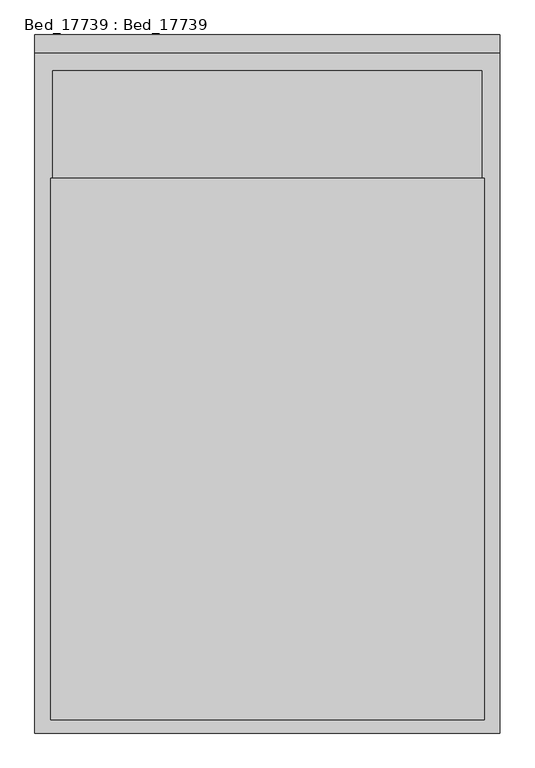
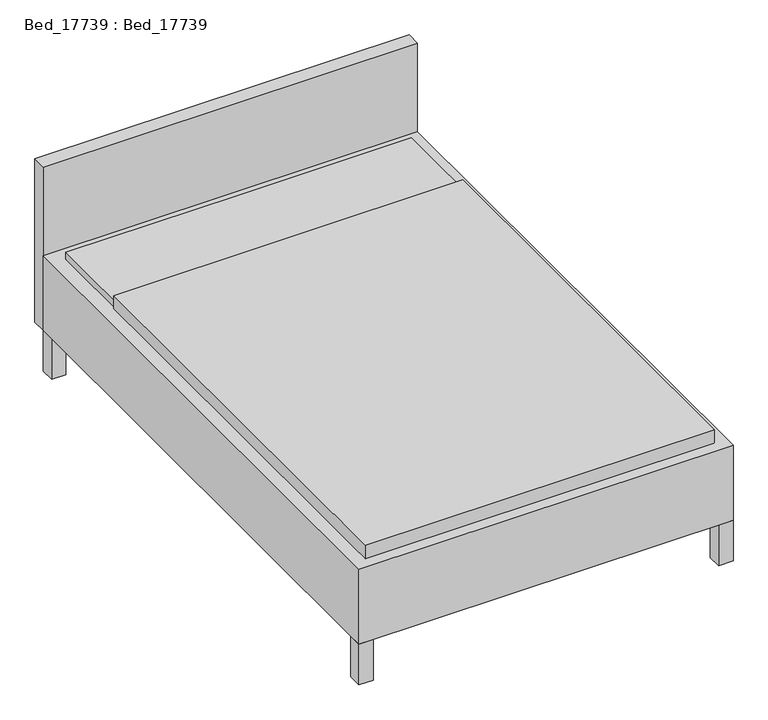
"""IFC4 building model written with IfcOpenShell, lengths in millimetres: furniture geometry, Bed_17739 : Bed_17739."""

from ifc_helpers import new_model, si_unit, frame, origin, origin_with_axes, place, context, project, spatial, polyline, outline, extrude, source, transform, mapped, element, save


def bed_17739_bed_17739_15c61121(model_context):
    return source(origin(), model_context, "Body", "SweptSolid", [
        extrude(outline(polyline([(-609.6, 914.4), (0.0, 914.4), (609.6, 914.4), (609.6, -914.4), (-609.6, -914.4), (-609.6, 0.0), (-609.6, 914.4)])), frame((0.0, 0.0, 152.4), z_axis=(0.0, 0.0, 1.0), x_axis=(1.0, 0.0, 0.0)), (0.0, 0.0, 1.0), 304.8),
        extrude(outline(polyline([(660.4, -965.2), (-660.4, -965.2), (-660.4, 965.2), (660.4, 965.2), (660.4, -965.2)]), holes=[polyline([(609.6, 914.4), (-609.6, 914.4), (-609.6, -914.4), (609.6, -914.4), (609.6, 914.4)])]), frame((0.0, 0.0, 152.4), z_axis=(0.0, 0.0, 1.0), x_axis=(1.0, 0.0, 0.0)), (0.0, 0.0, 1.0), 279.4),
        extrude(outline(polyline([(609.6, 914.4), (609.6, 965.2), (660.4, 965.2), (660.4, 914.4), (609.6, 914.4)])), origin_with_axes(), (0.0, 0.0, 1.0), 152.4),
        extrude(outline(polyline([(660.4, -914.4), (660.4, -965.2), (609.6, -965.2), (609.6, -914.4), (660.4, -914.4)])), origin_with_axes(), (0.0, 0.0, 1.0), 152.4),
        extrude(outline(polyline([(-609.6, -965.2), (-660.4, -965.2), (-660.4, -914.4), (-609.6, -914.4), (-609.6, -965.2)])), origin_with_axes(), (0.0, 0.0, 1.0), 152.4),
        extrude(outline(polyline([(-609.6, 914.4), (-660.4, 914.4), (-660.4, 965.2), (-609.6, 965.2), (-609.6, 914.4)])), origin_with_axes(), (0.0, 0.0, 1.0), 152.4),
        extrude(outline(polyline([(-660.4, 1016.0), (660.4, 1016.0), (660.4, 965.2), (-660.4, 965.2), (-660.4, 1016.0)])), frame((0.0, 0.0, 152.4), z_axis=(0.0, 0.0, 1.0), x_axis=(1.0, 0.0, 0.0)), (0.0, 0.0, 1.0), 609.6),
        extrude(outline(polyline([(615.95, 609.6), (615.95, -927.1), (-615.95, -927.1), (-615.95, 609.6), (615.95, 609.6)])), frame((0.0, 0.0, 431.8), z_axis=(0.0, 0.0, 1.0), x_axis=(1.0, 0.0, 0.0)), (0.0, 0.0, 1.0), 50.8),
    ])


if __name__ == "__main__":
    model = new_model("IFC4")
    model_context = context("Model", 3, world=origin())
    ifc_project = project(units=[si_unit("LENGTHUNIT", "METRE", prefix="MILLI")], contexts=[model_context])
    site = spatial("IfcSite", under=ifc_project)
    building = spatial("IfcBuilding", under=site)
    placement = place(None, origin())
    bed_17739_bed_17739_shape = bed_17739_bed_17739_15c61121(model_context)
    element("IfcFurniture", 1, ObjectType="Bed_17739 : Bed_17739", at=placement, inside=building, context=model_context, shape_type="MappedRepresentation", body=[
        mapped(bed_17739_bed_17739_shape, transform((0.0, 0.0, 0.0), x_axis=(1.0, 0.0, 0.0), y_axis=(0.0, 1.0, 0.0), z_axis=(0.0, 0.0, 1.0))),
    ])
    save(model, "model.ifc")

# Revit data of these elements
# Type "Bed_17739 : Bed_17739"
#   Default Elevation = 0
# Element 1 (IfcFurniture, "Bed_17739 : Bed_17739")
#   Materials on its faces: "legs", "sheets", "bed frame", "Blanket"
# Materials
#   "legs": colour RGB 90 73 37, transparency 0, Cost = 0
#   "sheets": colour RGB 200 195 176, transparency 0, Cost = 0
#   "bed frame": colour RGB 90 73 37, transparency 0, Cost = 0
#   "Blanket": class "System", colour RGB 59 0 1, transparency 0, Cost = 0
